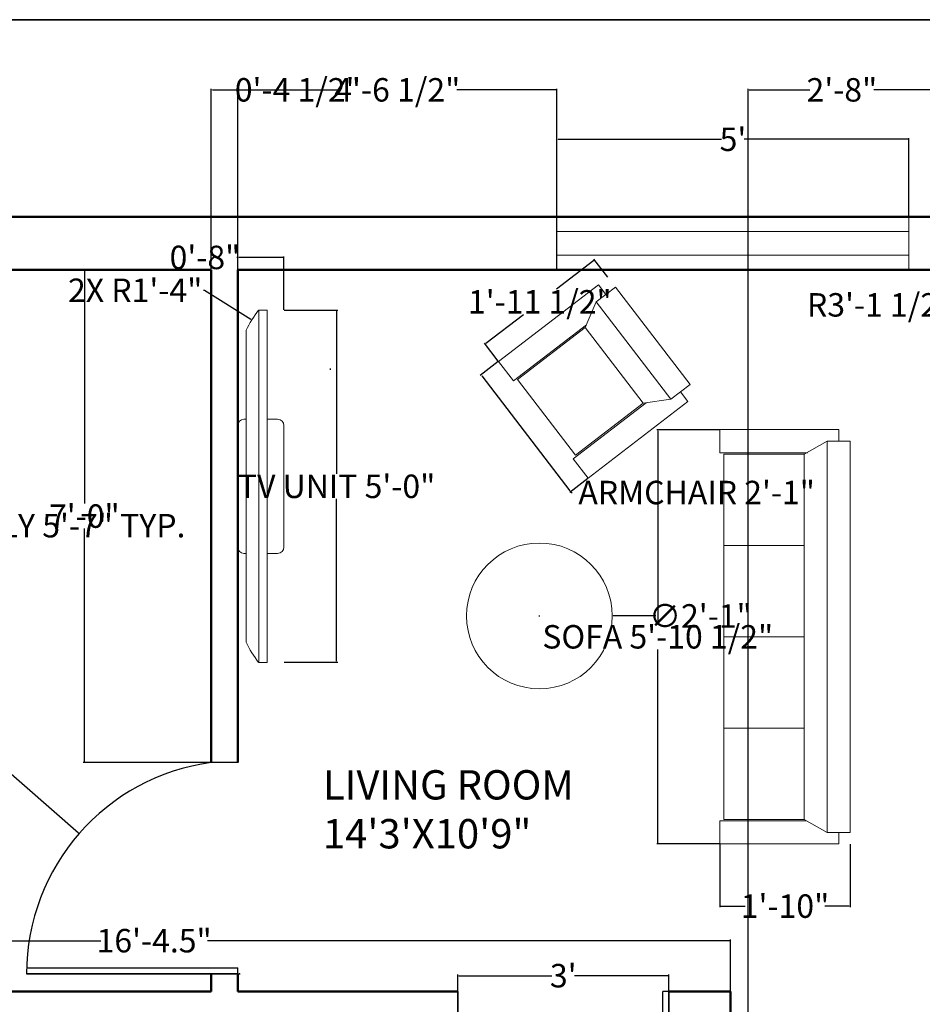
# Model space of a CAD drawing. Units: inches. Extents: x 124 to 591, y 365 to 713.
# Tile 4 of 5: x 264 to 418, y 545 to 713. Entities that reach past the tile are written whole.
import ezdxf

# ---------------------------------------------------------------- set-up
doc = ezdxf.new("R2010")
doc.units = ezdxf.units.IN
doc.header["$MEASUREMENT"] = 0
for name, color, linetype, lineweight in [('A-ANNO-DIMS', 2, 'Continuous', 18), ('A-ANNO-TTLB', 7, 'Continuous', 35), ('A-AREA-IDEN', 7, 'Continuous', 25), ('A-DOOR', 4, 'Continuous', 25), ('A-EQPM', 8, 'Continuous', 18), ('A-GLAZ', 4, 'Continuous', 18), ('A-WALL', 7, 'Continuous', 50), ('furniture', 8, 'Continuous', 13)]:
    doc.layers.add(name, color=color, linetype=linetype, lineweight=lineweight)
doc.styles.get("Standard").update_dxf_attribs({"font": 'arial.ttf'})
doc.dimstyles.get("Standard").update_dxf_attribs({"dimtxt": 4, "dimasz": 0.18, "dimexe": 0.18, "dimexo": 0.0625, "dimgap": 0.09, "dimtad": 0, "dimtih": 1, "dimtoh": 1, "dimdec": 1, "dimzin": 0, "dimdsep": 46, "dimlunit": 3, "dimtxsty": 'Standard', "dimcen": 0.09, "dimclrd": 6, "dimclrt": 3, "dimadec": 0, "dimazin": 0, "dimtfac": 1, "dimtdec": 1, "dimtofl": 0, "dimtmove": 0, "dimatfit": 3, "dimfxl": 1, "dimtfillclr": 6, "dimtolj": 1, "dimtzin": 0, "dimarcsym": 0})

# ---------------------------------------------------------------- blocks, each defined once
blk = doc.blocks.new('PLASMA-LARGE')
at = {"layer": 'furniture'}
for p, q in [((-7.26, 0), (7.26, 0)), ((-18.61, -1), (18.61, -1)), ((-8, -1), (-8, -0.74)), ((8, -1), (8, -0.74)), ((-21, -2.5), (21, -2.5)), ((-21, -2.5), (-21, -3.5)), ((-21, -3.5), (21, -3.5)), ((-8, -3.5), (-8, -4.76)), ((8, -3.5), (8, -4.76)), ((21, -2.5), (21, -3.5)), ((-7.26, -5.5), (7.26, -5.5))]:
    blk.add_line(p, q, dxfattribs=at)
for centre, radius, start, end in [((-7.26, -0.74), 0.744, 90, 180), ((7.26, -0.74), 0.744, 0, 90), ((-13.97, -11.05), 11.07, 114.7602, 129.4175), ((13.97, -11.05), 11.07, 50.5825, 65.2398), ((-7.26, -4.76), 0.744, 180, 270), ((7.26, -4.76), 0.744, 270, 0)]:
    blk.add_arc(centre, radius, start, end, dxfattribs=at)
blk = doc.blocks.new('FABRIC SOFA 4S')
at = {"layer": 'furniture'}
for p, q in [((3, 54), (34, 54)), ((3, 51), (3, 54)), ((34, 48), (34, 54)), ((0, -51), (0, 51)), ((6, 51), (0, 51)), ((6, -51), (6, 51)), ((12, 47.63), (6, 51)), ((11.14, 48), (34, 48)), ((33, 23.81), (12, 23.81)), ((33, 0), (12, 0)), ((33, -23.81), (12, -23.81)), ((6, -51), (12, -47.63)), ((11.54, -48), (34, -48)), ((34, -48), (34, -54)), ((6, -51), (0, -51)), ((3, -54), (3, -51)), ((3, -54), (34, -54))]:
    blk.add_line(p, q, dxfattribs=at)
blk.add_lwpolyline([(12, -47.63), (12, 47.63), (33, 47.63), (33, -47.63)], close=True, dxfattribs=at)
blk = doc.blocks.new('FABRIC SOFA 1S')
at = {"layer": 'furniture'}
for p, q in [((3, 18.12), (34, 18.12)), ((3, 15.12), (3, 18.12)), ((34, 12.12), (34, 18.12)), ((0, -15.12), (0, 15.12)), ((6, 15.12), (0, 15.12)), ((6, -15.12), (6, 15.12)), ((12, 11.75), (6, 15.12)), ((11.33, 12.12), (34, 12.12)), ((6, -15.12), (12, -11.75)), ((11.33, -12.12), (34, -12.12)), ((34, -12.12), (34, -18.12)), ((6, -15.12), (0, -15.12)), ((3, -18.12), (3, -15.12)), ((3, -18.12), (34, -18.12))]:
    blk.add_line(p, q, dxfattribs=at)
blk.add_lwpolyline([(12, -11.75), (12, 11.75), (33, 11.75), (33, -11.75)], close=True, dxfattribs=at)
blk = doc.blocks.new('*D21')
at = {"layer": 'A-ANNO-DIMS', "color": 0, "lineweight": -2, "transparency": 16777216}
for p, q in [((356.07, 679.15), (356.07, 692.5)), ((356.25, 692.32), (384.14, 692.32)), ((415.89, 692.32), (388, 692.32)), ((416.07, 679.15), (416.07, 692.5))]:
    blk.add_line(p, q, dxfattribs=at)
at = {"layer": 'A-ANNO-DIMS', "color": 0, "transparency": 16777216}
for points in [[(356.25, 692.35), (356.25, 692.29), (356.07, 692.32)], [(415.89, 692.35), (415.89, 692.29), (416.07, 692.32)]]:
    blk.add_solid(points, dxfattribs=at)
at = {"layer": 'Defpoints', "color": 0, "transparency": 16777216}
for p in [(416.07, 692.32), (356.07, 679.09), (416.07, 679.09)]:
    blk.add_point(p, dxfattribs=at)
at = {"layer": 'A-ANNO-DIMS', "color": 0, "transparency": 16777216, "insert": (386.07, 692.32), "char_height": 4, "attachment_point": 5}
blk.add_mtext("\\A1;5'", dxfattribs=at)
blk = doc.blocks.new('*D24')
at = {"layer": 'A-ANNO-DIMS', "color": 0, "lineweight": -2, "transparency": 16777216}
for p, q in [((189.14, 547.36), (189.14, 555.91)), ((189.32, 555.73), (278.29, 555.73)), ((385.46, 555.73), (296.49, 555.73)), ((385.64, 547.15), (385.64, 555.91))]:
    blk.add_line(p, q, dxfattribs=at)
at = {"layer": 'A-ANNO-DIMS', "color": 0, "transparency": 16777216}
for points in [[(189.32, 555.76), (189.32, 555.7), (189.14, 555.73)], [(385.46, 555.76), (385.46, 555.7), (385.64, 555.73)]]:
    blk.add_solid(points, dxfattribs=at)
at = {"layer": 'Defpoints', "color": 0, "transparency": 16777216}
for p in [(385.64, 555.73), (189.14, 547.3), (385.64, 547.09)]:
    blk.add_point(p, dxfattribs=at)
at = {"layer": 'A-ANNO-DIMS', "color": 0, "transparency": 16777216, "insert": (287.39, 555.73), "char_height": 4, "attachment_point": 5}
blk.add_mtext('\\A1;16\'-4.5"', dxfattribs=at)
blk = doc.blocks.new('*D25')
at = {"layer": 'A-ANNO-DIMS', "color": 0, "lineweight": -2, "transparency": 16777216}
for p, q in [((339.14, 542.65), (339.14, 549.94)), ((339.32, 549.76), (355.21, 549.76)), ((374.96, 549.76), (359.07, 549.76)), ((375.14, 542.65), (375.14, 549.94))]:
    blk.add_line(p, q, dxfattribs=at)
at = {"layer": 'A-ANNO-DIMS', "color": 0, "transparency": 16777216}
for points in [[(339.32, 549.79), (339.32, 549.73), (339.14, 549.76)], [(374.96, 549.79), (374.96, 549.73), (375.14, 549.76)]]:
    blk.add_solid(points, dxfattribs=at)
at = {"layer": 'Defpoints', "color": 0, "transparency": 16777216}
for p in [(375.14, 549.76), (339.14, 542.59), (375.14, 542.59)]:
    blk.add_point(p, dxfattribs=at)
at = {"layer": 'A-ANNO-DIMS', "color": 0, "transparency": 16777216, "insert": (357.14, 549.76), "char_height": 4, "attachment_point": 5}
blk.add_mtext("\\A1;3'", dxfattribs=at)
blk = doc.blocks.new('DOOR-SWING-36IN')
for p, q in [((36, 36), (31.5, 36)), ((0, 1), (36, 1)), ((36, 0), (36, 1)), ((36, 0), (0, 0)), ((0, 0), (36, 0))]:
    blk.add_line(p, q)
blk.add_arc((36.32, 0), 36.32, 97.6281, 180)
blk = doc.blocks.new('*D28')
at = {"layer": 'A-ANNO-DIMS', "color": 0, "lineweight": -2, "transparency": 16777216}
for p, q in [((250.53, 660.08), (260.74, 660.08)), ((250.53, 592.85), (260.74, 592.85))]:
    blk.add_line(p, q, dxfattribs=at)
at = {"layer": 'A-ANNO-DIMS', "color": 6, "lineweight": -2, "transparency": 16777216}
for p, q in [((260.56, 659.9), (260.56, 628.62)), ((260.56, 593.03), (260.56, 624.31))]:
    blk.add_line(p, q, dxfattribs=at)
at = {"layer": 'A-ANNO-DIMS', "color": 6, "transparency": 16777216}
for points in [[(260.53, 659.9), (260.59, 659.9), (260.56, 660.08)], [(260.53, 593.03), (260.59, 593.03), (260.56, 592.85)]]:
    blk.add_solid(points, dxfattribs=at)
at = {"layer": 'Defpoints', "color": 0, "transparency": 16777216}
for p in [(250.47, 660.08), (260.56, 660.08), (250.47, 592.85)]:
    blk.add_point(p, dxfattribs=at)
at = {"layer": 'A-ANNO-DIMS', "color": 3, "transparency": 16777216, "insert": (260.56, 626.46), "char_height": 4, "attachment_point": 5}
blk.add_mtext('\\A1;BED ASSEMBLY 5\'-7" TYP.', dxfattribs=at)
blk = doc.blocks.new('*D36')
at = {"layer": 'A-ANNO-DIMS', "color": 0, "lineweight": -2, "transparency": 16777216}
for p, q in [((309.56, 663.18), (318.68, 663.18)), ((309.56, 603.17), (318.68, 603.17))]:
    blk.add_line(p, q, dxfattribs=at)
at = {"layer": 'A-ANNO-DIMS', "color": 6, "lineweight": -2, "transparency": 16777216}
for p, q in [((318.5, 663), (318.5, 635.31)), ((318.5, 603.35), (318.5, 631.04))]:
    blk.add_line(p, q, dxfattribs=at)
at = {"layer": 'A-ANNO-DIMS', "color": 6, "transparency": 16777216}
for points in [[(318.47, 663), (318.53, 663), (318.5, 663.18)], [(318.47, 603.35), (318.53, 603.35), (318.5, 603.17)]]:
    blk.add_solid(points, dxfattribs=at)
at = {"layer": 'Defpoints', "color": 0, "transparency": 16777216}
for p in [(309.5, 663.18), (318.5, 663.18), (309.5, 603.17)]:
    blk.add_point(p, dxfattribs=at)
at = {"layer": 'A-ANNO-DIMS', "color": 3, "transparency": 16777216, "insert": (318.5, 633.17), "char_height": 4, "attachment_point": 5}
blk.add_mtext('\\A1;TV UNIT 5\'-0"', dxfattribs=at)
blk = doc.blocks.new('*D37')
at = {"layer": 'A-ANNO-DIMS', "color": 6, "lineweight": -2, "transparency": 16777216}
for p, q in [((301.64, 672.18), (301.46, 672.18)), ((309.32, 672.18), (301.82, 672.18))]:
    blk.add_line(p, q, dxfattribs=at)
at = {"layer": 'A-ANNO-DIMS', "color": 0, "lineweight": -2, "transparency": 16777216}
for p, q in [((301.64, 663.24), (301.64, 672.36)), ((309.5, 663.24), (309.5, 672.36))]:
    blk.add_line(p, q, dxfattribs=at)
at = {"layer": 'A-ANNO-DIMS', "color": 6, "transparency": 16777216}
for points in [[(301.82, 672.21), (301.82, 672.15), (301.64, 672.18)], [(309.32, 672.21), (309.32, 672.15), (309.5, 672.18)]]:
    blk.add_solid(points, dxfattribs=at)
at = {"layer": 'Defpoints', "color": 0, "transparency": 16777216}
for p in [(301.64, 672.18), (301.64, 663.18), (309.5, 663.18)]:
    blk.add_point(p, dxfattribs=at)
at = {"layer": 'A-ANNO-DIMS', "color": 3, "transparency": 16777216, "insert": (296.05, 672.18), "char_height": 4, "attachment_point": 5}
blk.add_mtext('\\A1;0\'-8"', dxfattribs=at)
blk = doc.blocks.new('*D40')
at = {"layer": 'A-ANNO-DIMS', "color": 0, "lineweight": -2, "transparency": 16777216}
for p, q in [((383.77, 642.82), (373.07, 642.82)), ((383.77, 572.21), (373.07, 572.21))]:
    blk.add_line(p, q, dxfattribs=at)
at = {"layer": 'A-ANNO-DIMS', "color": 6, "lineweight": -2, "transparency": 16777216}
for p, q in [((373.25, 642.64), (373.25, 609.68)), ((373.25, 572.39), (373.25, 605.36))]:
    blk.add_line(p, q, dxfattribs=at)
at = {"layer": 'A-ANNO-DIMS', "color": 6, "transparency": 16777216}
for points in [[(373.22, 642.64), (373.28, 642.64), (373.25, 642.82)], [(373.22, 572.39), (373.28, 572.39), (373.25, 572.21)]]:
    blk.add_solid(points, dxfattribs=at)
at = {"layer": 'Defpoints', "color": 0, "transparency": 16777216}
for p in [(373.25, 642.82), (383.84, 642.82), (383.84, 572.21)]:
    blk.add_point(p, dxfattribs=at)
at = {"layer": 'A-ANNO-DIMS', "color": 3, "transparency": 16777216, "insert": (373.25, 607.52), "char_height": 4, "attachment_point": 5}
blk.add_mtext('\\A1;SOFA 5\'-10 1/2"', dxfattribs=at)
blk = doc.blocks.new('*D41')
at = {"layer": 'A-ANNO-DIMS', "color": 0, "lineweight": -2, "transparency": 16777216}
for p, q in [((383.84, 572.15), (383.84, 561.44)), ((406.07, 572.15), (406.07, 561.44))]:
    blk.add_line(p, q, dxfattribs=at)
at = {"layer": 'A-ANNO-DIMS', "color": 6, "lineweight": -2, "transparency": 16777216}
for p, q in [((384.02, 561.62), (388.18, 561.62)), ((405.89, 561.62), (401.72, 561.62))]:
    blk.add_line(p, q, dxfattribs=at)
at = {"layer": 'A-ANNO-DIMS', "color": 6, "transparency": 16777216}
for points in [[(384.02, 561.65), (384.02, 561.59), (383.84, 561.62)], [(405.89, 561.65), (405.89, 561.59), (406.07, 561.62)]]:
    blk.add_solid(points, dxfattribs=at)
at = {"layer": 'Defpoints', "color": 0, "transparency": 16777216}
for p in [(383.84, 572.21), (406.07, 572.21), (383.84, 561.62)]:
    blk.add_point(p, dxfattribs=at)
at = {"layer": 'A-ANNO-DIMS', "color": 3, "transparency": 16777216, "insert": (394.95, 561.62), "char_height": 4, "attachment_point": 5}
blk.add_mtext('\\A1;1\'-10"', dxfattribs=at)
blk = doc.blocks.new('*D42')
at = {"layer": 'A-ANNO-DIMS', "color": 0, "lineweight": -2, "transparency": 16777216}
for p, q in [((346.05, 654.42), (342.97, 652.06)), ((361.33, 634.5), (358.25, 632.14))]:
    blk.add_line(p, q, dxfattribs=at)
at = {"layer": 'A-ANNO-DIMS', "color": 6, "lineweight": -2, "transparency": 16777216}
for p, q in [((343.23, 652.02), (358.28, 632.39)), ((358.39, 632.25), (358.5, 632.11)), ((358.5, 632.11), (358.68, 632.11))]:
    blk.add_line(p, q, dxfattribs=at)
at = {"layer": 'A-ANNO-DIMS', "color": 6, "transparency": 16777216}
for points in [[(343.25, 652.04), (343.2, 652.01), (343.12, 652.17)], [(358.3, 632.41), (358.26, 632.37), (358.39, 632.25)]]:
    blk.add_solid(points, dxfattribs=at)
at = {"layer": 'Defpoints', "color": 0, "transparency": 16777216}
for p in [(346.1, 654.46), (361.38, 634.54), (358.39, 632.25)]:
    blk.add_point(p, dxfattribs=at)
at = {"layer": 'A-ANNO-DIMS', "color": 3, "transparency": 16777216, "insert": (379.88, 632.11), "char_height": 4, "attachment_point": 5}
blk.add_mtext('\\A1;ARMCHAIR 2\'-1"', dxfattribs=at)
blk = doc.blocks.new('*D43')
at = {"layer": 'A-ANNO-DIMS', "color": 6, "lineweight": -2, "transparency": 16777216}
for p, q in [((362.35, 671.66), (355.97, 666.77)), ((343.96, 657.56), (350.34, 662.45))]:
    blk.add_line(p, q, dxfattribs=at)
at = {"layer": 'A-ANNO-DIMS', "color": 0, "lineweight": -2, "transparency": 16777216}
for p, q in [((364.75, 668.83), (362.38, 671.91)), ((346.07, 654.51), (343.7, 657.59))]:
    blk.add_line(p, q, dxfattribs=at)
at = {"layer": 'A-ANNO-DIMS', "color": 6, "transparency": 16777216}
for points in [[(362.33, 671.69), (362.37, 671.64), (362.49, 671.77)], [(343.94, 657.58), (343.97, 657.53), (343.81, 657.45)]]:
    blk.add_solid(points, dxfattribs=at)
at = {"layer": 'Defpoints', "color": 0, "transparency": 16777216}
for p in [(364.79, 668.78), (343.81, 657.45), (346.1, 654.46)]:
    blk.add_point(p, dxfattribs=at)
at = {"layer": 'A-ANNO-DIMS', "color": 3, "transparency": 16777216, "insert": (353.15, 664.61), "char_height": 4, "attachment_point": 5}
blk.add_mtext('\\A1;1\'-11 1/2"', dxfattribs=at)
blk = doc.blocks.new('*D48')
at = {"layer": 'A-ANNO-DIMS', "color": 0, "lineweight": -2, "transparency": 16777216}
for p, q in [((301.64, 670.15), (301.64, 700.92)), ((356.07, 670.15), (356.07, 700.92))]:
    blk.add_line(p, q, dxfattribs=at)
at = {"layer": 'A-ANNO-DIMS', "color": 6, "lineweight": -2, "transparency": 16777216}
for p, q in [((301.82, 700.74), (318.71, 700.74)), ((355.89, 700.74), (339, 700.74))]:
    blk.add_line(p, q, dxfattribs=at)
at = {"layer": 'A-ANNO-DIMS', "color": 6, "transparency": 16777216}
for points in [[(301.82, 700.77), (301.82, 700.71), (301.64, 700.74)], [(355.89, 700.77), (355.89, 700.71), (356.07, 700.74)]]:
    blk.add_solid(points, dxfattribs=at)
at = {"layer": 'Defpoints', "color": 0, "transparency": 16777216}
for p in [(356.07, 700.74), (301.64, 670.09), (356.07, 670.09)]:
    blk.add_point(p, dxfattribs=at)
at = {"layer": 'A-ANNO-DIMS', "color": 3, "transparency": 16777216, "insert": (328.85, 700.74), "char_height": 4, "attachment_point": 5}
blk.add_mtext('\\A1;4\'-6 1/2"', dxfattribs=at)
blk = doc.blocks.new('*D57')
at = {"layer": 'A-ANNO-DIMS', "color": 0, "lineweight": -2, "transparency": 16777216}
for p, q in [((388.64, 451.15), (388.64, 700.92)), ((420.64, 451.15), (420.64, 700.92))]:
    blk.add_line(p, q, dxfattribs=at)
at = {"layer": 'A-ANNO-DIMS', "color": 6, "lineweight": -2, "transparency": 16777216}
for p, q in [((388.82, 700.74), (399.2, 700.74)), ((420.46, 700.74), (410.08, 700.74))]:
    blk.add_line(p, q, dxfattribs=at)
at = {"layer": 'A-ANNO-DIMS', "color": 6, "transparency": 16777216}
for points in [[(388.82, 700.77), (388.82, 700.71), (388.64, 700.74)], [(420.46, 700.77), (420.46, 700.71), (420.64, 700.74)]]:
    blk.add_solid(points, dxfattribs=at)
at = {"layer": 'Defpoints', "color": 0, "transparency": 16777216}
for p in [(420.64, 700.74), (388.64, 451.09), (420.64, 451.09)]:
    blk.add_point(p, dxfattribs=at)
at = {"layer": 'A-ANNO-DIMS', "color": 3, "transparency": 16777216, "insert": (404.64, 700.74), "char_height": 4, "attachment_point": 5}
blk.add_mtext('\\A1;2\'-8"', dxfattribs=at)
blk = doc.blocks.new('*D59')
at = {"layer": 'A-ANNO-DIMS', "color": 0, "lineweight": -2, "transparency": 16777216}
for p, q in [((297.14, 670.15), (297.14, 700.92)), ((301.64, 670.15), (301.64, 700.92))]:
    blk.add_line(p, q, dxfattribs=at)
at = {"layer": 'A-ANNO-DIMS', "color": 6, "lineweight": -2, "transparency": 16777216}
for p, q in [((297.32, 700.74), (301.46, 700.74)), ((301.64, 700.74), (301.82, 700.74))]:
    blk.add_line(p, q, dxfattribs=at)
at = {"layer": 'A-ANNO-DIMS', "color": 6, "transparency": 16777216}
for points in [[(297.32, 700.77), (297.32, 700.71), (297.14, 700.74)], [(301.46, 700.77), (301.46, 700.71), (301.64, 700.74)]]:
    blk.add_solid(points, dxfattribs=at)
at = {"layer": 'Defpoints', "color": 0, "transparency": 16777216}
for p in [(301.64, 700.74), (297.14, 670.09), (301.64, 670.09)]:
    blk.add_point(p, dxfattribs=at)
at = {"layer": 'A-ANNO-DIMS', "color": 3, "transparency": 16777216, "insert": (311.88, 700.74), "char_height": 4, "attachment_point": 5}
blk.add_mtext('\\A1;0\'-4 1/2"', dxfattribs=at)
blk = doc.blocks.new('*D61')
at = {"layer": 'A-ANNO-DIMS', "color": 0, "lineweight": -2, "transparency": 16777216}
for p, q in [((297.08, 670.09), (275.31, 670.09)), ((297.08, 586.09), (275.31, 586.09))]:
    blk.add_line(p, q, dxfattribs=at)
at = {"layer": 'A-ANNO-DIMS', "color": 6, "lineweight": -2, "transparency": 16777216}
for p, q in [((275.49, 669.91), (275.49, 630.22)), ((275.49, 586.27), (275.49, 625.96))]:
    blk.add_line(p, q, dxfattribs=at)
at = {"layer": 'A-ANNO-DIMS', "color": 6, "transparency": 16777216}
for points in [[(275.46, 669.91), (275.52, 669.91), (275.49, 670.09)], [(275.46, 586.27), (275.52, 586.27), (275.49, 586.09)]]:
    blk.add_solid(points, dxfattribs=at)
at = {"layer": 'Defpoints', "color": 0, "transparency": 16777216}
for p in [(275.49, 670.09), (297.14, 670.09), (297.14, 586.09)]:
    blk.add_point(p, dxfattribs=at)
at = {"layer": 'A-ANNO-DIMS', "color": 3, "transparency": 16777216, "insert": (275.49, 628.09), "char_height": 4, "attachment_point": 5}
blk.add_mtext('\\A1;7\'-0"', dxfattribs=at)
blk = doc.blocks.new('*D67')
at = {"layer": 'A-ANNO-DIMS', "color": 0, "lineweight": -2, "transparency": 16777216}
for p, q in [((352.98, 611.08), (353.16, 611.08)), ((353.07, 610.99), (353.07, 611.17))]:
    blk.add_line(p, q, dxfattribs=at)
at = {"layer": 'A-ANNO-DIMS', "color": 6, "lineweight": -2, "transparency": 16777216}
blk.add_line((372.94, 611.08), (365.67, 611.08), dxfattribs=at)
at = {"layer": 'A-ANNO-DIMS', "color": 6, "transparency": 16777216}
blk.add_solid([(365.67, 611.11), (365.67, 611.05), (365.49, 611.08)], dxfattribs=at)
at = {"layer": 'Defpoints', "color": 0, "transparency": 16777216}
for p in [(340.65, 611.08), (365.49, 611.08)]:
    blk.add_point(p, dxfattribs=at)
at = {"layer": 'A-ANNO-DIMS', "color": 3, "transparency": 16777216, "insert": (380.52, 611.08), "char_height": 4, "attachment_point": 5}
blk.add_mtext('\\A1;∅2\'-1"', dxfattribs=at)
blk = doc.blocks.new('*D68')
at = {"layer": 'A-ANNO-DIMS', "color": 6, "lineweight": -2, "transparency": 16777216}
for p, q in [((258.04, 588.36), (258.22, 588.36)), ((258.22, 588.36), (274.49, 574.13))]:
    blk.add_line(p, q, dxfattribs=at)
at = {"layer": 'A-ANNO-DIMS', "color": 0, "lineweight": -2, "transparency": 16777216}
for p, q in [((301.87, 550.09), (302.05, 550.09)), ((301.96, 550), (301.96, 550.18))]:
    blk.add_line(p, q, dxfattribs=at)
at = {"layer": 'A-ANNO-DIMS', "color": 6, "transparency": 16777216}
blk.add_solid([(274.51, 574.15), (274.47, 574.11), (274.62, 574.01)], dxfattribs=at)
at = {"layer": 'Defpoints', "color": 0, "transparency": 16777216}
for p in [(274.62, 574.01), (301.96, 550.09)]:
    blk.add_point(p, dxfattribs=at)
at = {"layer": 'A-ANNO-DIMS', "color": 3, "transparency": 16777216, "insert": (241.73, 588.36), "char_height": 4, "attachment_point": 5}
blk.add_mtext('\\A1;2X R3\'-0 1/2"', dxfattribs=at)
blk = doc.blocks.new('*D71')
at = {"layer": 'A-ANNO-DIMS', "color": 6, "lineweight": -2, "transparency": 16777216}
blk.add_line((423.14, 664.09), (445.46, 664.09), dxfattribs=at)
at = {"layer": 'A-ANNO-DIMS', "color": 0, "lineweight": -2, "transparency": 16777216}
for p, q in [((483.05, 664.09), (483.23, 664.09)), ((483.14, 664), (483.14, 664.18))]:
    blk.add_line(p, q, dxfattribs=at)
at = {"layer": 'A-ANNO-DIMS', "color": 6, "transparency": 16777216}
blk.add_solid([(445.46, 664.12), (445.46, 664.06), (445.64, 664.09)], dxfattribs=at)
at = {"layer": 'Defpoints', "color": 0, "transparency": 16777216}
for p in [(445.64, 664.09), (483.14, 664.09)]:
    blk.add_point(p, dxfattribs=at)
at = {"layer": 'A-ANNO-DIMS', "color": 3, "transparency": 16777216, "insert": (411.16, 664.09), "char_height": 4, "attachment_point": 5}
blk.add_mtext('\\A1;R3\'-1 1/2"', dxfattribs=at)
blk = doc.blocks.new('*D74')
at = {"layer": 'A-ANNO-DIMS', "color": 6, "lineweight": -2, "transparency": 16777216}
for p, q in [((295.81, 666.58), (295.99, 666.58)), ((295.99, 666.58), (303.88, 661.63))]:
    blk.add_line(p, q, dxfattribs=at)
at = {"layer": 'A-ANNO-DIMS', "color": 0, "lineweight": -2, "transparency": 16777216}
for p, q in [((317.34, 653.14), (317.52, 653.14)), ((317.43, 653.05), (317.43, 653.23))]:
    blk.add_line(p, q, dxfattribs=at)
at = {"layer": 'A-ANNO-DIMS', "color": 6, "transparency": 16777216}
blk.add_solid([(303.89, 661.66), (303.86, 661.61), (304.03, 661.54)], dxfattribs=at)
at = {"layer": 'Defpoints', "color": 0, "transparency": 16777216}
for p in [(304.03, 661.54), (317.43, 653.14)]:
    blk.add_point(p, dxfattribs=at)
at = {"layer": 'A-ANNO-DIMS', "color": 3, "transparency": 16777216, "insert": (284.16, 666.58), "char_height": 4, "attachment_point": 5}
blk.add_mtext('\\A1;2X R1\'-4"', dxfattribs=at)

msp = doc.modelspace()

# ---------------------------------------------------------------- linework, layer by layer
at = {"layer": 'A-ANNO-TTLB'}
msp.add_lwpolyline([(124.09, 712.7), (590.57, 712.7), (590.57, 365.95), (124.09, 365.95)], close=True, dxfattribs=at)
msp.add_lwpolyline([(124.09, 712.7), (590.57, 712.7), (590.57, 365.95), (124.09, 365.95)], close=True, dxfattribs=at)
at = {"layer": 'A-GLAZ'}
for p, q in [((356.07, 674.59), (356.07, 679.09)), ((356.07, 679.09), (356.07, 670.09)), ((416.07, 679.09), (416.07, 670.09)), ((416.07, 676.59), (356.07, 676.59)), ((416.07, 670.09), (416.07, 674.59)), ((416.07, 672.59), (356.07, 672.59))]:
    msp.add_line(p, q, dxfattribs=at)
at = {"layer": 'A-WALL'}
for p, q in [((180.14, 679.09), (562.14, 679.09)), ((189.14, 670.09), (297.14, 670.09)), ((297.14, 670.09), (297.14, 586.09)), ((301.64, 670.09), (301.64, 586.09)), ((301.64, 670.09), (472.64, 670.09)), ((297.14, 550.09), (297.14, 547.09)), ((301.64, 547.09), (301.64, 550.09)), ((301.64, 550.09), (301.64, 547.09)), ((189.14, 547.09), (297.14, 547.09)), ((301.64, 547.09), (339.14, 547.09)), ((381.14, 547.09), (375.14, 547.09)), ((375.14, 547.09), (385.64, 547.09)), ((385.64, 547.09), (385.64, 451.09))]:
    msp.add_line(p, q, dxfattribs=at)
at = {"layer": 'furniture'}
msp.add_circle((353.07, 611.08), 12.42, dxfattribs=at)

# ---------------------------------------------------------------- block references
at = {"layer": 'A-DOOR'}
msp.add_blockref('DOOR-SWING-36IN', (265.64, 550.09), dxfattribs=at)
at = {"layer": 'A-DOOR', "rotation": 89.99999999999976}
msp.add_blockref('DOOR-SWING-36IN', (375.14, 511.09), dxfattribs=at)
at = {"layer": 'A-EQPM', "xscale": 1.42874999999896, "yscale": 1.42874999999896, "zscale": 1.42874999999896, "rotation": 90}
msp.add_blockref('PLASMA-LARGE', (301.64, 633.17), dxfattribs=at)
at = {"layer": 'furniture'}
for name, p, xscale, yscale, zscale, rotation in [('FABRIC SOFA 1S', (372.42, 658.83), 0.6924093716078898, 0.6924093716078898, 0.6924093716078898, 217.4827598044174), ('FABRIC SOFA 4S', (406.07, 607.52), -0.6537939928824033, 0.6537939928824033, 0.6537939928824033, 359.999999999979)]:
    msp.add_blockref(name, p, dxfattribs=dict(at, xscale=xscale, yscale=yscale, zscale=zscale, rotation=rotation))

# ---------------------------------------------------------------- texts
at = {"layer": 'A-AREA-IDEN', "insert": (316.17, 584.79), "char_height": 5, "attachment_point": 1}
msp.add_mtext_dynamic_manual_height_columns('LIVING ROOM\\P14\'3\'X10\'9"', width=53.8845, gutter_width=1, heights=[0], dxfattribs=at)

# ---------------------------------------------------------------- dimensions: what is measured, and where the dimension line sits
at = {"layer": 'A-ANNO-DIMS'}
for base, p1, p2, override, picture, middle in [((301.64, 700.74), (297.14, 670.09), (301.64, 670.09), {"dimdec": 1, "dimlfac": 1, "dimrnd": 0, "dimzin": 1, "dimdsep": 46, "dimlunit": 4, "dimfrac": 2}, '*D59', (311.88, 700.74)), ((356.07, 700.74), (301.64, 670.09), (356.07, 670.09), {"dimdec": 1, "dimlfac": 1, "dimrnd": 0, "dimzin": 1, "dimdsep": 46, "dimlunit": 4, "dimfrac": 2}, '*D48', (328.85, 700.74)), ((420.64, 700.74), (388.64, 451.09), (420.64, 451.09), {"dimdec": 1, "dimlfac": 1, "dimrnd": 0, "dimzin": 1, "dimdsep": 46, "dimlunit": 4, "dimfrac": 2}, '*D57', (404.64, 700.74)), ((416.07, 692.32), (356.07, 679.09), (416.07, 679.09), {"dimclrd": 0, "dimclre": 0, "dimclrt": 0}, '*D21', (386.07, 692.32)), ((385.64, 555.73), (189.14, 547.3), (385.64, 547.09), {"dimclrd": 0, "dimclre": 0, "dimclrt": 0}, '*D24', (287.39, 555.73)), ((375.14, 549.76), (339.14, 542.59), (375.14, 542.59), {"dimclrd": 0, "dimclre": 0, "dimclrt": 0}, '*D25', (357.14, 549.76))]:
    dim = msp.add_linear_dim(base=base, p1=p1, p2=p2, dimstyle='Standard', override=override, dxfattribs=at)
    dim.commit()
    dim.dimension.update_dxf_attribs({"geometry": picture, "text_midpoint": middle})
for base, p1, p2, angle, picture, middle in [((301.64, 672.18), (309.5, 663.18), (301.64, 663.18), 180, '*D37', (296.05, 672.18)), ((343.81, 657.45), (364.79, 668.78), (346.1, 654.46), 217.4828, '*D43', (353.15, 664.61)), ((275.49, 670.09), (297.14, 586.09), (297.14, 670.09), 90, '*D61', (275.49, 628.09)), ((383.84, 561.62), (406.07, 572.21), (383.84, 572.21), 180, '*D41', (394.95, 561.62))]:
    dim = msp.add_linear_dim(base=base, p1=p1, p2=p2, angle=angle, dimstyle='Standard', override={"dimdec": 1, "dimlfac": 1, "dimrnd": 0, "dimzin": 1, "dimdsep": 46, "dimlunit": 4, "dimfrac": 2}, dxfattribs=at)
    dim.commit()
    dim.dimension.update_dxf_attribs({"geometry": picture, "text_midpoint": middle})
for center, mpoint, picture, middle in [((317.43, 653.14), (304.03, 661.54), '*D74', (284.16, 666.58)), ((301.96, 550.09), (274.62, 574.01), '*D68', (241.73, 588.36))]:
    dim = msp.add_radius_dim(center=center, mpoint=mpoint, text='2X <>', dimstyle='Standard', override={"dimdec": 1, "dimlfac": 1, "dimrnd": 0, "dimzin": 1, "dimdsep": 46, "dimlunit": 4, "dimfrac": 2}, dxfattribs=at)
    dim.commit()
    dim.dimension.update_dxf_attribs({"geometry": picture, "text_midpoint": middle, "dimtype": 164})
dim = msp.add_radius_dim(center=(483.14, 664.09), mpoint=(445.64, 664.09), dimstyle='Standard', override={"dimdec": 1, "dimlfac": 1, "dimrnd": 0, "dimzin": 1, "dimdsep": 46, "dimlunit": 4, "dimfrac": 2}, dxfattribs=at)
dim.commit()
dim.dimension.update_dxf_attribs({"geometry": '*D71', "text_midpoint": (423.14, 664.09), "dimtype": 164})
for base, p1, p2, angle, text, picture, middle in [((318.5, 663.18), (309.5, 603.17), (309.5, 663.18), 90, 'TV UNIT <>', '*D36', (318.5, 633.17)), ((260.56, 660.08), (250.47, 592.85), (250.47, 660.08), 90, 'BED ASSEMBLY <> TYP.', '*D28', (260.56, 626.46)), ((358.39, 632.25), (346.1, 654.46), (361.38, 634.54), 307.4828, 'ARMCHAIR <>', '*D42', (379.88, 632.11)), ((373.25, 642.82), (383.84, 572.21), (383.84, 642.82), 90, 'SOFA <>', '*D40', (373.25, 607.52))]:
    dim = msp.add_linear_dim(base=base, p1=p1, p2=p2, angle=angle, text=text, dimstyle='Standard', override={"dimdec": 1, "dimlfac": 1, "dimrnd": 0, "dimzin": 1, "dimdsep": 46, "dimlunit": 4, "dimfrac": 2}, dxfattribs=at)
    dim.commit()
    dim.dimension.update_dxf_attribs({"geometry": picture, "text_midpoint": middle})
dim = msp.add_diameter_dim_2p(p1=(340.65, 611.08), p2=(365.49, 611.08), dimstyle='Standard', override={"dimdec": 1, "dimlfac": 1, "dimrnd": 0, "dimzin": 1, "dimdsep": 46, "dimlunit": 4, "dimfrac": 2}, dxfattribs=at)
dim.commit()
dim.dimension.update_dxf_attribs({"geometry": '*D67', "text_midpoint": (372.94, 611.08), "dimtype": 163})

doc.saveas('drawing.dxf')
